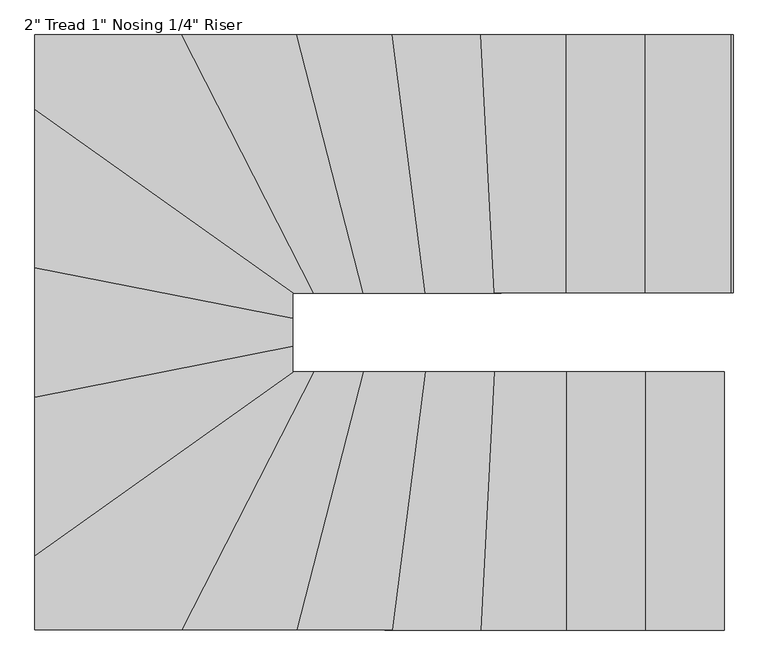
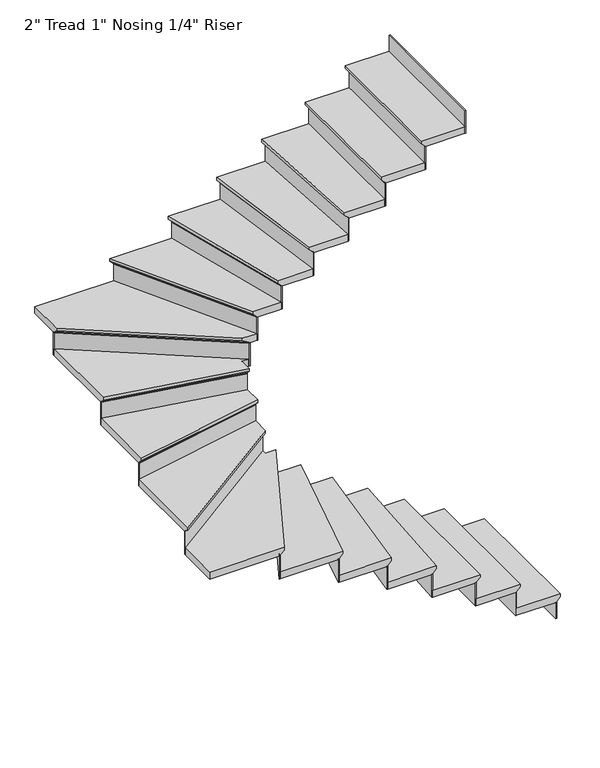
"""IFC4 building model written with IfcOpenShell, lengths in millimetres: stair flight geometry."""

from ifc_helpers import new_model, si_unit, origin, place, context, project, spatial, faceted_brep, source, transform, mapped, element, save


def stair_flight_f6e367ce(model_context):
    return source(origin(), model_context, "Body", "Brep", [
        faceted_brep([(-9800.0917773, 2757.4116886, 150.2833333), (-9800.0917773, 2757.4116886, 169.3333333), (-9800.0917773, 1843.0116886, 169.3333333), (-9800.0917773, 1843.0116886, 150.2833333), (-9825.4917773, 2757.4116886, 124.8833333), (-9825.4917773, 1843.0116886, 124.8833333), (-10104.8917773, 2757.4116886, 169.3333333), (-10104.8917773, 1843.0116886, 169.3333333), (-9825.4917773, 1843.0116886, 118.5333333), (-10104.8917773, 1843.0116886, 118.5333333), (-10104.8917773, 2757.4116886, 118.5333333), (-9825.4917773, 2757.4116886, 118.5333333)], [[[0, 1, 2, 3]], [[4, 0, 3, 5]], [[2, 1, 6, 7]], [[8, 9, 10, 11]], [[2, 7, 9, 8, 5, 3]], [[8, 11, 4, 5]], [[6, 1, 0, 4, 11, 10]], [[7, 6, 10, 9]]]),
        faceted_brep([(-9825.4917773, 2757.4116886, 118.5333333), (-9825.4917773, 2757.4116886, 0.0), (-9831.8417773, 2757.4116886, 0.0), (-9831.8417773, 2757.4116886, 118.5333333), (-9825.4917773, 1843.0116886, 118.5333333), (-9831.8417773, 1843.0116886, 118.5333333), (-9831.8417773, 1843.0116886, 0.0), (-9825.4917773, 1843.0116886, 0.0)], [[[0, 1, 2, 3]], [[4, 5, 6, 7]], [[1, 0, 4, 7]], [[2, 1, 7, 6]], [[3, 2, 6, 5]], [[0, 3, 5, 4]]]),
        faceted_brep([(-10104.8917773, 2757.4116886, 287.8666667), (-10104.8917773, 2757.4116886, 118.5333333), (-10111.2417773, 2757.4116886, 118.5333333), (-10111.2417773, 2757.4116886, 287.8666667), (-10104.8917773, 1843.0116886, 287.8666667), (-10111.2417773, 1843.0116886, 287.8666667), (-10111.2417773, 1843.0116886, 118.5333333), (-10104.8917773, 1843.0116886, 118.5333333)], [[[0, 1, 2, 3]], [[4, 5, 6, 7]], [[1, 0, 4, 7]], [[2, 1, 7, 6]], [[3, 2, 6, 5]], [[0, 3, 5, 4]]]),
        faceted_brep([(-10079.4917773, 1843.0116886, 338.6666667), (-10079.4917773, 2757.4116886, 338.6666667), (-10384.2917773, 2757.4116886, 338.6666667), (-10384.2917773, 1843.0116886, 338.6666667), (-10104.8917773, 1843.0116886, 287.8666667), (-10384.2917773, 1843.0116886, 287.8666667), (-10384.2917773, 2757.4116886, 287.8666667), (-10104.8917773, 2757.4116886, 287.8666667), (-10104.8917773, 1843.0116886, 294.2166667), (-10079.4917773, 1843.0116886, 319.6166667), (-10104.8917773, 2757.4116886, 294.2166667), (-10079.4917773, 2757.4116886, 319.6166667)], [[[0, 1, 2, 3]], [[4, 5, 6, 7]], [[0, 3, 5, 4, 8, 9]], [[4, 7, 10, 8]], [[2, 1, 11, 10, 7, 6]], [[3, 2, 6, 5]], [[11, 1, 0, 9]], [[10, 11, 9, 8]]]),
        faceted_brep([(-10384.2917773, 2757.4116886, 457.2), (-10384.2917773, 2757.4116886, 287.8666667), (-10390.6417773, 2757.4116886, 287.8666667), (-10390.6417773, 2757.4116886, 457.2), (-10384.2917773, 1843.0116886, 457.2), (-10390.6417773, 1843.0116886, 457.2), (-10390.6417773, 1843.0116886, 287.8666667), (-10384.2917773, 1843.0116886, 287.8666667)], [[[0, 1, 2, 3]], [[4, 5, 6, 7]], [[1, 0, 4, 7]], [[2, 1, 7, 6]], [[3, 2, 6, 5]], [[0, 3, 5, 4]]]),
        faceted_brep([(-10358.8917773, 1843.0116886, 508.0), (-10358.8917773, 2757.4116886, 508.0), (-10639.9589388, 2757.4116886, 508.0), (-10687.4932092, 1843.0116886, 508.0), (-10384.2917773, 1843.0116886, 457.2), (-10687.4932092, 1843.0116886, 457.2), (-10639.9589388, 2757.4116886, 457.2), (-10384.2917773, 2757.4116886, 457.2), (-10384.2917773, 1843.0116886, 463.55), (-10358.8917773, 1843.0116886, 488.95), (-10384.2917773, 2757.4116886, 463.55), (-10358.8917773, 2757.4116886, 488.95)], [[[0, 1, 2, 3]], [[4, 5, 6, 7]], [[0, 3, 5, 4, 8, 9]], [[4, 7, 10, 8]], [[2, 1, 11, 10, 7, 6]], [[3, 2, 6, 5]], [[11, 1, 0, 9]], [[10, 11, 9, 8]]]),
        faceted_brep([(-10639.9589388, 2757.4116886, 626.5333333), (-10639.9589388, 2757.4116886, 457.2), (-10646.3175129, 2757.4116886, 457.2), (-10646.3175129, 2757.4116886, 626.5333333), (-10687.4932092, 1843.0116886, 626.5333333), (-10693.8517833, 1843.0116886, 626.5333333), (-10693.8517833, 1843.0116886, 457.2), (-10687.4932092, 1843.0116886, 457.2)], [[[0, 1, 2, 3]], [[4, 5, 6, 7]], [[1, 0, 4, 7]], [[2, 1, 7, 6]], [[3, 2, 6, 5]], [[0, 3, 5, 4]]]),
        faceted_brep([(-10662.0589125, 1843.0116886, 677.3333333), (-10614.5246421, 2757.4116886, 677.3333333), (-10884.1256386, 2757.4116886, 677.3333333), (-11002.4816902, 1843.0116886, 677.3333333), (-10687.4932092, 1843.0116886, 626.5333333), (-11002.4816902, 1843.0116886, 626.5333333), (-10884.1256386, 2757.4116886, 626.5333333), (-10639.9589388, 2757.4116886, 626.5333333), (-10687.4932092, 1843.0116886, 632.8833333), (-10662.0589125, 1843.0116886, 658.2833333), (-10639.9589388, 2757.4116886, 632.8833333), (-10614.5246421, 2757.4116886, 658.2833333)], [[[0, 1, 2, 3]], [[4, 5, 6, 7]], [[0, 3, 5, 4, 8, 9]], [[4, 7, 10, 8]], [[2, 1, 11, 10, 7, 6]], [[3, 2, 6, 5]], [[11, 1, 0, 9]], [[10, 11, 9, 8]]]),
        faceted_brep([(-10884.1256386, 2757.4116886, 795.8666667), (-10884.1256386, 2757.4116886, 626.5333333), (-10890.5286104, 2757.4116886, 626.5333333), (-10890.5286104, 2757.4116886, 795.8666667), (-11002.4816902, 1843.0116886, 795.8666667), (-11008.884662, 1843.0116886, 795.8666667), (-11008.884662, 1843.0116886, 626.5333333), (-11002.4816902, 1843.0116886, 626.5333333)], [[[0, 1, 2, 3]], [[4, 5, 6, 7]], [[1, 0, 4, 7]], [[2, 1, 7, 6]], [[3, 2, 6, 5]], [[0, 3, 5, 4]]]),
        faceted_brep([(-10976.8698031, 1843.0116886, 846.6666667), (-10858.5137515, 2757.4116886, 846.6666667), (-11105.7528611, 2757.4116886, 846.6666667), (-11340.8833085, 1843.0116886, 846.6666667), (-11002.4816902, 1843.0116886, 795.8666667), (-11340.8833085, 1843.0116886, 795.8666667), (-11105.7528611, 2757.4116886, 795.8666667), (-10884.1256386, 2757.4116886, 795.8666667), (-11002.4816902, 1843.0116886, 802.2166667), (-10976.8698031, 1843.0116886, 827.6166667), (-10884.1256386, 2757.4116886, 802.2166667), (-10858.5137515, 2757.4116886, 827.6166667)], [[[0, 1, 2, 3]], [[4, 5, 6, 7]], [[0, 3, 5, 4, 8, 9]], [[4, 7, 10, 8]], [[2, 1, 11, 10, 7, 6]], [[3, 2, 6, 5]], [[11, 1, 0, 9]], [[10, 11, 9, 8]]]),
        faceted_brep([(-11105.7528611, 2757.4116886, 965.2), (-11105.7528611, 2757.4116886, 795.8666667), (-11112.3094379, 2757.4116886, 795.8666667), (-11112.3094379, 2757.4116886, 965.2), (-11340.8833085, 1843.0116886, 965.2), (-11347.4398853, 1843.0116886, 965.2), (-11347.4398853, 1843.0116886, 795.8666667), (-11340.8833085, 1843.0116886, 795.8666667)], [[[0, 1, 2, 3]], [[4, 5, 6, 7]], [[1, 0, 4, 7]], [[2, 1, 7, 6]], [[3, 2, 6, 5]], [[0, 3, 5, 4]]]),
        faceted_brep([(-11314.657001, 1843.0116886, 1016.0), (-11079.5265536, 2757.4116886, 1016.0), (-11282.0994971, 2757.4116886, 1016.0), (-11750.9241185, 1843.0116886, 1016.0), (-11340.8833085, 1843.0116886, 965.2), (-11750.9241185, 1843.0116886, 965.2), (-11282.0994971, 2757.4116886, 965.2), (-11105.7528611, 2757.4116886, 965.2), (-11340.8833085, 1843.0116886, 971.55), (-11314.657001, 1843.0116886, 996.95), (-11105.7528611, 2757.4116886, 971.55), (-11079.5265536, 2757.4116886, 996.95)], [[[0, 1, 2, 3]], [[4, 5, 6, 7]], [[0, 3, 5, 4, 8, 9]], [[4, 7, 10, 8]], [[2, 1, 11, 10, 7, 6]], [[3, 2, 6, 5]], [[11, 1, 0, 9]], [[10, 11, 9, 8]]]),
        faceted_brep([(-11282.0994971, 2757.4116886, 1134.5333333), (-11282.0994971, 2757.4116886, 965.2), (-11289.2354803, 2757.4116886, 965.2), (-11289.2354803, 2757.4116886, 1134.5333333), (-11750.9241185, 1843.0116886, 1134.5333333), (-11758.0601016, 1843.0116886, 1134.5333333), (-11758.0601016, 1843.0116886, 965.2), (-11750.9241185, 1843.0116886, 965.2)], [[[0, 1, 2, 3]], [[4, 5, 6, 7]], [[1, 0, 4, 7]], [[2, 1, 7, 6]], [[3, 2, 6, 5]], [[0, 3, 5, 4]]]),
        faceted_brep([(-12242.2234692, 2136.6928223, 1185.3333333), (-12242.2234692, 1843.0116886, 1185.3333333), (-11722.3801859, 1843.0116886, 1185.3333333), (-11253.5555646, 2757.4116886, 1185.3333333), (-11327.8234692, 2757.4116886, 1185.3333333), (-11327.8234692, 2786.9667715, 1185.3333333), (-12242.2234692, 1843.0116886, 1134.5333333), (-12242.2234692, 2136.6928223, 1134.5333333), (-11327.8234692, 2786.9667715, 1134.5333333), (-11327.8234692, 2757.4116886, 1134.5333333), (-11282.0994971, 2757.4116886, 1134.5333333), (-11750.9241185, 1843.0116886, 1134.5333333), (-11750.9241185, 1843.0116886, 1140.8833333), (-11722.3801859, 1843.0116886, 1166.2833333), (-11282.0994971, 2757.4116886, 1140.8833333), (-11253.5555646, 2757.4116886, 1166.2833333)], [[[0, 1, 2, 3, 4, 5]], [[6, 7, 8, 9, 10, 11]], [[1, 0, 7, 6]], [[2, 1, 6, 11, 12, 13]], [[11, 10, 14, 12]], [[4, 3, 15, 14, 10, 9]], [[5, 4, 9, 8]], [[0, 5, 8, 7]], [[15, 3, 2, 13]], [[14, 15, 13, 12]]]),
        faceted_brep([(-11327.8234692, 2786.9667715, 1303.8666667), (-11327.8234692, 2786.9667715, 1134.5333333), (-11327.8234692, 2794.7587463, 1134.5333333), (-11327.8234692, 2794.7587463, 1303.8666667), (-12242.2234692, 2136.6928223, 1303.8666667), (-12242.2234692, 2144.4847971, 1303.8666667), (-12242.2234692, 2144.4847971, 1134.5333333), (-12242.2234692, 2136.6928223, 1134.5333333)], [[[0, 1, 2, 3]], [[4, 5, 6, 7]], [[1, 0, 4, 7]], [[2, 1, 7, 6]], [[3, 2, 6, 5]], [[0, 3, 5, 4]]]),
        faceted_brep([(-12242.2234692, 2105.5249231, 1354.6666667), (-11327.8234692, 2755.7988723, 1354.6666667), (-11327.8234692, 2873.4208585, 1354.6666667), (-12242.2234692, 2693.1800022, 1354.6666667), (-12242.2234692, 2136.6928223, 1303.8666667), (-12242.2234692, 2693.1800022, 1303.8666667), (-11327.8234692, 2873.4208585, 1303.8666667), (-11327.8234692, 2786.9667715, 1303.8666667), (-12242.2234692, 2136.6928223, 1310.2166667), (-12242.2234692, 2105.5249231, 1335.6166667), (-11327.8234692, 2786.9667715, 1310.2166667), (-11327.8234692, 2755.7988723, 1335.6166667)], [[[0, 1, 2, 3]], [[4, 5, 6, 7]], [[0, 3, 5, 4, 8, 9]], [[4, 7, 10, 8]], [[2, 1, 11, 10, 7, 6]], [[3, 2, 6, 5]], [[11, 1, 0, 9]], [[10, 11, 9, 8]]]),
        faceted_brep([(-11327.8234692, 2873.4208585, 1473.2), (-11327.8234692, 2873.4208585, 1303.8666667), (-11327.8234692, 2879.893044, 1303.8666667), (-11327.8234692, 2879.893044, 1473.2), (-12242.2234692, 2693.1800022, 1473.2), (-12242.2234692, 2699.6521876, 1473.2), (-12242.2234692, 2699.6521876, 1303.8666667), (-12242.2234692, 2693.1800022, 1303.8666667)], [[[0, 1, 2, 3]], [[4, 5, 6, 7]], [[1, 0, 4, 7]], [[2, 1, 7, 6]], [[3, 2, 6, 5]], [[0, 3, 5, 4]]]),
        faceted_brep([(-12242.2234692, 2667.2912605, 1524.0), (-11327.8234692, 2847.5321168, 1524.0), (-11327.8234692, 2972.5800022, 1524.0), (-12242.2234692, 3152.8208585, 1524.0), (-12242.2234692, 2693.1800022, 1473.2), (-12242.2234692, 3152.8208585, 1473.2), (-11327.8234692, 2972.5800022, 1473.2), (-11327.8234692, 2873.4208585, 1473.2), (-12242.2234692, 2693.1800022, 1479.55), (-12242.2234692, 2667.2912605, 1504.95), (-11327.8234692, 2873.4208585, 1479.55), (-11327.8234692, 2847.5321168, 1504.95)], [[[0, 1, 2, 3]], [[4, 5, 6, 7]], [[0, 3, 5, 4, 8, 9]], [[4, 7, 10, 8]], [[2, 1, 11, 10, 7, 6]], [[3, 2, 6, 5]], [[11, 1, 0, 9]], [[10, 11, 9, 8]]]),
        faceted_brep([(-11327.8234692, 2972.5800022, 1642.5333333), (-11327.8234692, 2972.5800022, 1473.2), (-11327.8234692, 2979.0521876, 1473.2), (-11327.8234692, 2979.0521876, 1642.5333333), (-12242.2234692, 3152.8208585, 1642.5333333), (-12242.2234692, 3159.293044, 1642.5333333), (-12242.2234692, 3159.293044, 1473.2), (-12242.2234692, 3152.8208585, 1473.2)], [[[0, 1, 2, 3]], [[4, 5, 6, 7]], [[1, 0, 4, 7]], [[2, 1, 7, 6]], [[3, 2, 6, 5]], [[0, 3, 5, 4]]]),
        faceted_brep([(-12242.2234692, 3126.9321168, 1693.3333333), (-11327.8234692, 2946.6912605, 1693.3333333), (-11327.8234692, 3036.8116886, 1693.3333333), (-11281.7279946, 3036.8116886, 1693.3333333), (-12242.2234692, 3719.8663533, 1693.3333333), (-12242.2234692, 3152.8208585, 1642.5333333), (-12242.2234692, 3719.8663533, 1642.5333333), (-11281.7279946, 3036.8116886, 1642.5333333), (-11327.8234692, 3036.8116886, 1642.5333333), (-11327.8234692, 2972.5800022, 1642.5333333), (-12242.2234692, 3152.8208585, 1648.8833333), (-12242.2234692, 3126.9321168, 1674.2833333), (-11327.8234692, 2972.5800022, 1648.8833333), (-11327.8234692, 2946.6912605, 1674.2833333)], [[[0, 1, 2, 3, 4]], [[5, 6, 7, 8, 9]], [[0, 4, 6, 5, 10, 11]], [[5, 9, 12, 10]], [[2, 1, 13, 12, 9, 8]], [[3, 2, 8, 7]], [[4, 3, 7, 6]], [[13, 1, 0, 11]], [[12, 13, 11, 10]]]),
        faceted_brep([(-11281.7279946, 3036.8116886, 1811.8666667), (-11281.7279946, 3036.8116886, 1642.5333333), (-11270.7711021, 3036.8116886, 1642.5333333), (-11270.7711021, 3036.8116886, 1811.8666667), (-12242.2234692, 3719.8663533, 1811.8666667), (-12242.2234692, 3727.6583281, 1811.8666667), (-12242.2234692, 3727.6583281, 1642.5333333), (-12242.2234692, 3719.8663533, 1642.5333333)], [[[0, 1, 2, 3]], [[4, 5, 6, 7]], [[1, 0, 4, 7]], [[2, 1, 7, 6]], [[3, 2, 6, 5]], [[0, 3, 5, 4]]]),
        faceted_brep([(-11693.8362534, 3951.2116886, 1862.6666667), (-12242.2234692, 3951.2116886, 1862.6666667), (-12242.2234692, 3688.6984541, 1862.6666667), (-11325.5555646, 3036.8116886, 1862.6666667), (-11225.0116321, 3036.8116886, 1862.6666667), (-12242.2234692, 3951.2116886, 1811.8666667), (-11693.8362534, 3951.2116886, 1811.8666667), (-11225.0116321, 3036.8116886, 1811.8666667), (-11281.7279946, 3036.8116886, 1811.8666667), (-12242.2234692, 3719.8663533, 1811.8666667), (-12242.2234692, 3719.8663533, 1818.2166667), (-12242.2234692, 3688.6984541, 1843.6166667), (-11281.7279946, 3036.8116886, 1818.2166667), (-11325.5555646, 3036.8116886, 1843.6166667)], [[[0, 1, 2, 3, 4]], [[5, 6, 7, 8, 9]], [[1, 0, 6, 5]], [[2, 1, 5, 9, 10, 11]], [[9, 8, 12, 10]], [[4, 3, 13, 12, 8, 7]], [[0, 4, 7, 6]], [[13, 3, 2, 11]], [[12, 13, 11, 10]]]),
        faceted_brep([(-11225.0116321, 3036.8116886, 1981.2), (-11225.0116321, 3036.8116886, 1811.8666667), (-11217.8756489, 3036.8116886, 1811.8666667), (-11217.8756489, 3036.8116886, 1981.2), (-11693.8362534, 3951.2116886, 1981.2), (-11686.7002703, 3951.2116886, 1981.2), (-11686.7002703, 3951.2116886, 1811.8666667), (-11693.8362534, 3951.2116886, 1811.8666667)], [[[0, 1, 2, 3]], [[4, 5, 6, 7]], [[1, 0, 4, 7]], [[2, 1, 7, 6]], [[3, 2, 6, 5]], [[0, 3, 5, 4]]]),
        faceted_brep([(-11722.3801859, 3951.2116886, 2032.0), (-11253.5555646, 3036.8116886, 2032.0), (-11053.3002461, 3036.8116886, 2032.0), (-11288.4306935, 3951.2116886, 2032.0), (-11693.8362534, 3951.2116886, 1981.2), (-11288.4306935, 3951.2116886, 1981.2), (-11053.3002461, 3036.8116886, 1981.2), (-11225.0116321, 3036.8116886, 1981.2), (-11693.8362534, 3951.2116886, 1987.55), (-11722.3801859, 3951.2116886, 2012.95), (-11225.0116321, 3036.8116886, 1987.55), (-11253.5555646, 3036.8116886, 2012.95)], [[[0, 1, 2, 3]], [[4, 5, 6, 7]], [[0, 3, 5, 4, 8, 9]], [[4, 7, 10, 8]], [[2, 1, 11, 10, 7, 6]], [[3, 2, 6, 5]], [[11, 1, 0, 9]], [[10, 11, 9, 8]]]),
        faceted_brep([(-11053.3002461, 3036.8116886, 2150.5333333), (-11053.3002461, 3036.8116886, 1981.2), (-11046.7436693, 3036.8116886, 1981.2), (-11046.7436693, 3036.8116886, 2150.5333333), (-11288.4306935, 3951.2116886, 2150.5333333), (-11281.8741167, 3951.2116886, 2150.5333333), (-11281.8741167, 3951.2116886, 1981.2), (-11288.4306935, 3951.2116886, 1981.2)], [[[0, 1, 2, 3]], [[4, 5, 6, 7]], [[1, 0, 4, 7]], [[2, 1, 7, 6]], [[3, 2, 6, 5]], [[0, 3, 5, 4]]]),
        faceted_brep([(-11314.657001, 3951.2116886, 2201.3333333), (-11079.5265536, 3036.8116886, 2201.3333333), (-10832.9018643, 3036.8116886, 2201.3333333), (-10951.257916, 3951.2116886, 2201.3333333), (-11288.4306935, 3951.2116886, 2150.5333333), (-10951.257916, 3951.2116886, 2150.5333333), (-10832.9018643, 3036.8116886, 2150.5333333), (-11053.3002461, 3036.8116886, 2150.5333333), (-11288.4306935, 3951.2116886, 2156.8833333), (-11314.657001, 3951.2116886, 2182.2833333), (-11053.3002461, 3036.8116886, 2156.8833333), (-11079.5265536, 3036.8116886, 2182.2833333)], [[[0, 1, 2, 3]], [[4, 5, 6, 7]], [[0, 3, 5, 4, 8, 9]], [[4, 7, 10, 8]], [[2, 1, 11, 10, 7, 6]], [[3, 2, 6, 5]], [[11, 1, 0, 9]], [[10, 11, 9, 8]]]),
        faceted_brep([(-10832.9018643, 3036.8116886, 2319.8666667), (-10832.9018643, 3036.8116886, 2150.5333333), (-10826.4988926, 3036.8116886, 2150.5333333), (-10826.4988926, 3036.8116886, 2319.8666667), (-10951.257916, 3951.2116886, 2319.8666667), (-10944.8549442, 3951.2116886, 2319.8666667), (-10944.8549442, 3951.2116886, 2150.5333333), (-10951.257916, 3951.2116886, 2150.5333333)], [[[0, 1, 2, 3]], [[4, 5, 6, 7]], [[1, 0, 4, 7]], [[2, 1, 7, 6]], [[3, 2, 6, 5]], [[0, 3, 5, 4]]]),
        faceted_brep([(-10976.8698031, 3951.2116886, 2370.6666667), (-10858.5137515, 3036.8116886, 2370.6666667), (-10589.0903454, 3036.8116886, 2370.6666667), (-10636.6246158, 3951.2116886, 2370.6666667), (-10951.257916, 3951.2116886, 2319.8666667), (-10636.6246158, 3951.2116886, 2319.8666667), (-10589.0903454, 3036.8116886, 2319.8666667), (-10832.9018643, 3036.8116886, 2319.8666667), (-10951.257916, 3951.2116886, 2326.2166667), (-10976.8698031, 3951.2116886, 2351.6166667), (-10832.9018643, 3036.8116886, 2326.2166667), (-10858.5137515, 3036.8116886, 2351.6166667)], [[[0, 1, 2, 3]], [[4, 5, 6, 7]], [[0, 3, 5, 4, 8, 9]], [[4, 7, 10, 8]], [[2, 1, 11, 10, 7, 6]], [[3, 2, 6, 5]], [[11, 1, 0, 9]], [[10, 11, 9, 8]]]),
        faceted_brep([(-10589.0903454, 3036.8116886, 2489.2), (-10589.0903454, 3036.8116886, 2319.8666667), (-10582.7317713, 3036.8116886, 2319.8666667), (-10582.7317713, 3036.8116886, 2489.2), (-10636.6246158, 3951.2116886, 2489.2), (-10630.2660417, 3951.2116886, 2489.2), (-10630.2660417, 3951.2116886, 2319.8666667), (-10636.6246158, 3951.2116886, 2319.8666667)], [[[0, 1, 2, 3]], [[4, 5, 6, 7]], [[1, 0, 4, 7]], [[2, 1, 7, 6]], [[3, 2, 6, 5]], [[0, 3, 5, 4]]]),
        faceted_brep([(-10662.0589125, 3951.2116886, 2540.0), (-10614.5246421, 3036.8116886, 2540.0), (-10333.4917773, 3036.8116886, 2540.0), (-10333.4917773, 3951.2116886, 2540.0), (-10636.6246158, 3951.2116886, 2489.2), (-10333.4917773, 3951.2116886, 2489.2), (-10333.4917773, 3036.8116886, 2489.2), (-10589.0903454, 3036.8116886, 2489.2), (-10636.6246158, 3951.2116886, 2495.55), (-10662.0589125, 3951.2116886, 2520.95), (-10589.0903454, 3036.8116886, 2495.55), (-10614.5246421, 3036.8116886, 2520.95)], [[[0, 1, 2, 3]], [[4, 5, 6, 7]], [[0, 3, 5, 4, 8, 9]], [[4, 7, 10, 8]], [[2, 1, 11, 10, 7, 6]], [[3, 2, 6, 5]], [[11, 1, 0, 9]], [[10, 11, 9, 8]]]),
        faceted_brep([(-10333.4917773, 3036.8116886, 2658.5333333), (-10333.4917773, 3036.8116886, 2489.2), (-10327.1417773, 3036.8116886, 2489.2), (-10327.1417773, 3036.8116886, 2658.5333333), (-10333.4917773, 3951.2116886, 2658.5333333), (-10327.1417773, 3951.2116886, 2658.5333333), (-10327.1417773, 3951.2116886, 2489.2), (-10333.4917773, 3951.2116886, 2489.2)], [[[0, 1, 2, 3]], [[4, 5, 6, 7]], [[1, 0, 4, 7]], [[2, 1, 7, 6]], [[3, 2, 6, 5]], [[0, 3, 5, 4]]]),
        faceted_brep([(-10358.8917773, 3951.2116886, 2709.3333333), (-10358.8917773, 3036.8116886, 2709.3333333), (-10054.0917773, 3036.8116886, 2709.3333333), (-10054.0917773, 3951.2116886, 2709.3333333), (-10333.4917773, 3951.2116886, 2658.5333333), (-10054.0917773, 3951.2116886, 2658.5333333), (-10054.0917773, 3036.8116886, 2658.5333333), (-10333.4917773, 3036.8116886, 2658.5333333), (-10333.4917773, 3951.2116886, 2664.8833333), (-10358.8917773, 3951.2116886, 2690.2833333), (-10333.4917773, 3036.8116886, 2664.8833333), (-10358.8917773, 3036.8116886, 2690.2833333)], [[[0, 1, 2, 3]], [[4, 5, 6, 7]], [[0, 3, 5, 4, 8, 9]], [[4, 7, 10, 8]], [[2, 1, 11, 10, 7, 6]], [[3, 2, 6, 5]], [[11, 1, 0, 9]], [[10, 11, 9, 8]]]),
        faceted_brep([(-10054.0917773, 3036.8116886, 2827.8666667), (-10054.0917773, 3036.8116886, 2658.5333333), (-10047.7417773, 3036.8116886, 2658.5333333), (-10047.7417773, 3036.8116886, 2827.8666667), (-10054.0917773, 3951.2116886, 2827.8666667), (-10047.7417773, 3951.2116886, 2827.8666667), (-10047.7417773, 3951.2116886, 2658.5333333), (-10054.0917773, 3951.2116886, 2658.5333333)], [[[0, 1, 2, 3]], [[4, 5, 6, 7]], [[1, 0, 4, 7]], [[2, 1, 7, 6]], [[3, 2, 6, 5]], [[0, 3, 5, 4]]]),
        faceted_brep([(-9774.6917773, 3036.8116886, 2997.2), (-9774.6917773, 3036.8116886, 2827.8666667), (-9768.3417773, 3036.8116886, 2827.8666667), (-9768.3417773, 3036.8116886, 2997.2), (-9774.6917773, 3951.2116886, 2997.2), (-9768.3417773, 3951.2116886, 2997.2), (-9768.3417773, 3951.2116886, 2827.8666667), (-9774.6917773, 3951.2116886, 2827.8666667)], [[[0, 1, 2, 3]], [[4, 5, 6, 7]], [[1, 0, 4, 7]], [[2, 1, 7, 6]], [[3, 2, 6, 5]], [[0, 3, 5, 4]]]),
        faceted_brep([(-10079.4917773, 3951.2116886, 2878.6666667), (-10079.4917773, 3036.8116886, 2878.6666667), (-9774.6917773, 3036.8116886, 2878.6666667), (-9774.6917773, 3951.2116886, 2878.6666667), (-10054.0917773, 3951.2116886, 2827.8666667), (-9774.6917773, 3951.2116886, 2827.8666667), (-9774.6917773, 3036.8116886, 2827.8666667), (-10054.0917773, 3036.8116886, 2827.8666667), (-10054.0917773, 3951.2116886, 2834.2166667), (-10079.4917773, 3951.2116886, 2859.6166667), (-10054.0917773, 3036.8116886, 2834.2166667), (-10079.4917773, 3036.8116886, 2859.6166667)], [[[0, 1, 2, 3]], [[4, 5, 6, 7]], [[0, 3, 5, 4, 8, 9]], [[4, 7, 10, 8]], [[2, 1, 11, 10, 7, 6]], [[3, 2, 6, 5]], [[11, 1, 0, 9]], [[10, 11, 9, 8]]]),
    ])


if __name__ == "__main__":
    model = new_model("IFC4")
    model_context = context("Model", 3, world=origin())
    ifc_project = project(units=[si_unit("LENGTHUNIT", "METRE", prefix="MILLI")], contexts=[model_context])
    site = spatial("IfcSite", under=ifc_project)
    building = spatial("IfcBuilding", under=site)
    placement = place(None, origin())
    stair_flight_shape = stair_flight_f6e367ce(model_context)
    element("IfcStairFlight", 1, ObjectType="2\" Tread 1\" Nosing 1/4\" Riser", at=placement, inside=building, context=model_context, shape_type="MappedRepresentation", body=[
        mapped(stair_flight_shape, transform((0.0, 0.0, 0.0), x_axis=(1.0, 0.0, 0.0), y_axis=(0.0, 1.0, 0.0), z_axis=(0.0, 0.0, 1.0))),
    ])
    save(model, "model.ifc")
